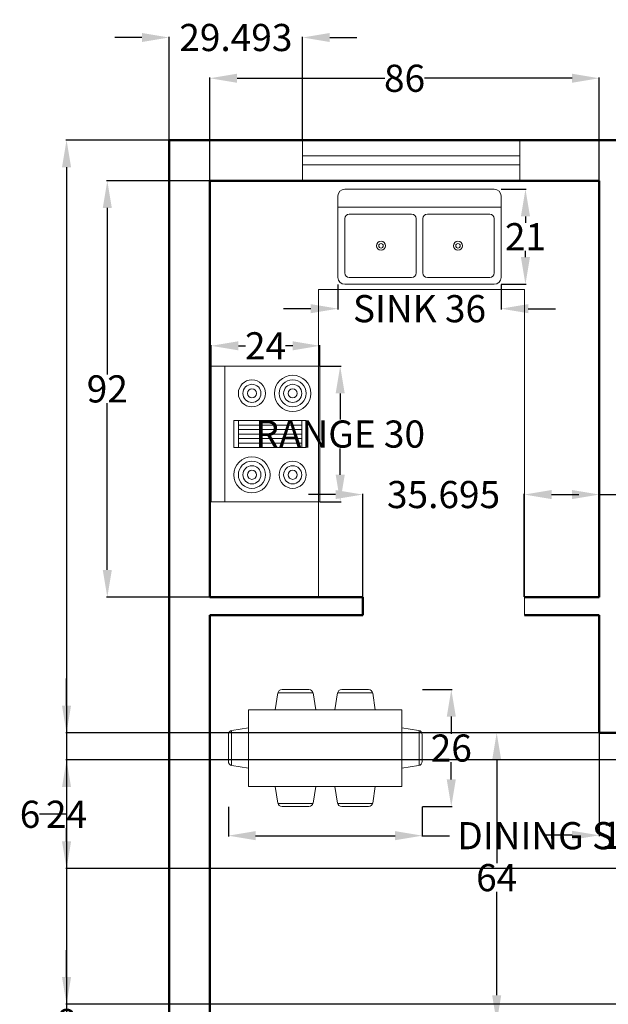
# Model space of a CAD drawing. Units: inches. Extents: x -8 to 300, y -428 to 46.
# Tile 3 of 4: x -8 to 122, y -172 to 46. Entities that reach past the tile are written whole.
import ezdxf

# ---------------------------------------------------------------- set-up
doc = ezdxf.new("R2010")
doc.units = ezdxf.units.IN
doc.header["$MEASUREMENT"] = 0
for name, color, linetype, lineweight in [('A-ANNO-DIMS', 2, 'Continuous', 18), ('A-EQPM', 8, 'Continuous', 18), ('A-FLOR-CASE', 9, 'Continuous', 18), ('A-FLOR-FIXT', 9, 'Continuous', 18), ('A-FURN', 8, 'Continuous', 18), ('A-GLAZ', 4, 'Continuous', 18), ('A-WALL', 7, 'Continuous', 50)]:
    doc.layers.add(name, color=color, linetype=linetype, lineweight=lineweight)
doc.styles.get("Standard").update_dxf_attribs({"font": 'arial.ttf'})
doc.dimstyles.get("Standard").update_dxf_attribs({"dimtxt": 6, "dimasz": 6, "dimexe": 0.18, "dimexo": 0.0625, "dimgap": 0.09, "dimtad": 0, "dimtih": 1, "dimtoh": 1, "dimdec": 0, "dimzin": 0, "dimdsep": 46, "dimlunit": 4, "dimtxsty": 'Standard', "dimcen": 0.09, "dimadec": 0, "dimazin": 0, "dimtfac": 1, "dimtdec": 0, "dimtofl": 0, "dimtmove": 0, "dimatfit": 3, "dimfxl": 1, "dimtolj": 1, "dimtzin": 0, "dimarcsym": 0})

# ---------------------------------------------------------------- blocks, each defined once
blk = doc.blocks.new('Dining Set - 36 x 72 in.')
for p, q in [((-22.23, 26), (-23.48, 18)), ((-22.23, 26), (-5.76, 26)), ((-5.84, 26.5), (-5.84, 26.5)), ((-4.52, 18), (-5.77, 26)), ((5.77, 26), (4.52, 18)), ((5.77, 26), (22.24, 26)), ((22.16, 26.5), (22.16, 26.5)), ((36, 18), (-36, 18)), ((-36, 18), (-36, -18)), ((36, -18), (36, 18)), ((-43.81, 8.26), (-36, 9.48)), ((43.81, 8.26), (36, 9.48)), ((-45.5, 6.29), (-45.5, -6.29)), ((-44, 8.23), (-44, -8.24)), ((44, 8.23), (44, -8.24)), ((45.5, 6.29), (45.5, -6.29)), ((-44.5, -8.16), (-44.5, -8.16)), ((-36, -9.48), (-43.81, -8.26)), ((36, -9.48), (43.81, -8.26)), ((44.5, -8.16), (44.5, -8.16)), ((-36, -18), (36, -18)), ((-22.26, -25.81), (-23.48, -18)), ((-4.52, -18), (-5.74, -25.81)), ((5.74, -25.81), (4.52, -18)), ((23.48, -18), (22.26, -25.81)), ((-22.23, -26), (-5.76, -26)), ((-20.29, -27.5), (-7.71, -27.5)), ((-5.84, -26.5), (-5.84, -26.5)), ((5.77, -26), (22.24, -26)), ((7.71, -27.5), (20.29, -27.5)), ((22.16, -26.5), (22.16, -26.5))]:
    blk.add_line(p, q)
for points in [[(-5.77, 26), (-5.74, 25.81, 0.369509), (-7.71, 27.5), (-20.28, 27.5, 0.370247), (-22.26, 25.8), (-22.23, 26)], [(5.7, 25.61), (5.74, 25.81, -0.369509), (7.71, 27.5), (20.29, 27.5, -0.36951), (22.26, 25.81), (23.48, 18)]]:
    blk.add_lwpolyline(points, format="xyb")
for centre, start, end in [((-43.5, 6.29), 98.8806, 180), ((43.5, 6.29), 0, 81.1194), ((-43.5, -6.29), 180, 261.1194), ((43.5, -6.29), 278.8806, 0), ((-20.29, -25.5), 188.8802, 270), ((-7.71, -25.5), 270, 351.1191), ((7.71, -25.5), 188.8802, 270), ((20.29, -25.5), 270, 351.1191)]:
    blk.add_arc(centre, 2, start, end)
blk = doc.blocks.new('Range-Oven - 30 in top')
for p, q in [((0, -3), (30, -3)), ((12, -6), (18, -6)), ((13, -20), (13, -6)), ((14, -6), (14, -20)), ((15, -20), (15, -6)), ((16, -6), (16, -20)), ((17, -20), (17, -6)), ((18, -20), (12, -20))]:
    blk.add_line(p, q)
for points in [[(0, -24), (0, 0), (30, 0), (30, -24)], [(12, -21), (12, -5), (18, -5), (18, -21)]]:
    blk.add_lwpolyline(points, close=True)
for centre, radius in [((6, -9), 4), ((6, -9), 3), ((24, -9), 3), ((6, -9), 2), ((6, -9), 1), ((24, -9), 2), ((24, -9), 1), ((6, -18), 3), ((24, -18), 4), ((24, -18), 3), ((6, -18), 2), ((6, -18), 1), ((24, -18), 2), ((24, -18), 1)]:
    blk.add_circle(centre, radius)
blk = doc.blocks.new('Sink-double - 36 in top')
for p, q in [((-18, -4), (18, -4)), ((-0.75, -18.5), (-0.75, -6.5)), ((0.75, -6.5), (0.75, -18.5))]:
    blk.add_line(p, q)
for points in [[(-16.5, 0), (16.5, 0)], [(-18, -19.5), (-18, -1.5)], [(18, -1.5), (18, -19.5)], [(-16.5, -18.5), (-16.5, -6.5)], [(-15.5, -5.5), (-1.75, -5.5)], [(1.75, -5.5), (15.5, -5.5)], [(16.5, -6.5), (16.5, -18.5)], [(-1.75, -19.5), (-15.5, -19.5)], [(15.5, -19.5), (1.75, -19.5)], [(16.5, -21), (-16.5, -21)]]:
    blk.add_lwpolyline(points)
for centre, radius in [((-8.5, -12.5), 1), ((-8.5, -12.5), 0.5), ((8.5, -12.5), 1), ((8.5, -12.5), 0.5)]:
    blk.add_circle(centre, radius)
for centre, radius, start, end in [((-16.5, -1.5), 1.5, 90, 180), ((16.5, -1.5), 1.5, 0, 90), ((-15.5, -6.5), 1, 90, 180), ((-1.75, -6.5), 1, 0, 90), ((1.75, -6.5), 1, 90, 180), ((15.5, -6.5), 1, 0, 90), ((-16.5, -19.5), 1.5, 180, 270), ((-15.5, -18.5), 1, 180, 270), ((-1.75, -18.5), 1, 270, 0), ((1.75, -18.5), 1, 180, 270), ((15.5, -18.5), 1, 270, 0), ((16.5, -19.5), 1.5, 270, 0)]:
    blk.add_arc(centre, radius, start, end)
blk = doc.blocks.new('*D23')
at = {"layer": 'A-ANNO-DIMS', "color": 0, "lineweight": -2, "transparency": 16777216}
for p, q in [((37.97, -128.08), (37.97, -134.62)), ((80.78, -128.08), (80.78, -134.62)), ((43.97, -134.44), (74.78, -134.44)), ((80.78, -134.44), (86.78, -134.44))]:
    blk.add_line(p, q, dxfattribs=at)
at = {"layer": 'A-ANNO-DIMS', "color": 0, "transparency": 16777216}
for points in [[(43.97, -133.44), (43.97, -135.44), (37.97, -134.44)], [(74.78, -133.44), (74.78, -135.44), (80.78, -134.44)]]:
    blk.add_solid(points, dxfattribs=at)
at = {"layer": 'Defpoints', "color": 0, "transparency": 16777216}
for p in [(37.97, -128.02), (80.78, -128.02), (80.78, -134.44)]:
    blk.add_point(p, dxfattribs=at)
at = {"layer": 'A-ANNO-DIMS', "color": 0, "transparency": 16777216, "insert": (116.16, -134.44), "char_height": 6, "attachment_point": 5}
blk.add_mtext('\\A1;DINING SET 43', dxfattribs=at)
blk = doc.blocks.new('*D24')
at = {"layer": 'A-ANNO-DIMS', "color": 0, "lineweight": -2, "transparency": 16777216}
for p, q in [((80.84, -102.14), (87.38, -102.14)), ((87.2, -108.14), (87.2, -111.93)), ((87.2, -122.02), (87.2, -118.23)), ((80.84, -128.02), (87.38, -128.02))]:
    blk.add_line(p, q, dxfattribs=at)
at = {"layer": 'A-ANNO-DIMS', "color": 0, "transparency": 16777216}
for points in [[(86.2, -108.14), (88.2, -108.14), (87.2, -102.14)], [(86.2, -122.02), (88.2, -122.02), (87.2, -128.02)]]:
    blk.add_solid(points, dxfattribs=at)
at = {"layer": 'Defpoints', "color": 0, "transparency": 16777216}
for p in [(80.78, -102.14), (87.2, -102.14), (80.78, -128.02)]:
    blk.add_point(p, dxfattribs=at)
at = {"layer": 'A-ANNO-DIMS', "color": 0, "transparency": 16777216, "insert": (87.2, -115.08), "char_height": 6, "attachment_point": 5}
blk.add_mtext('\\A1;26', dxfattribs=at)
blk = doc.blocks.new('*D25')
at = {"layer": 'A-ANNO-DIMS', "color": 0, "lineweight": -2, "transparency": 16777216}
for p, q in [((58.23, -30.69), (62.85, -30.69)), ((62.67, -36.69), (62.67, -42.5)), ((62.67, -54.69), (62.67, -48.89)), ((58.23, -60.69), (62.85, -60.69))]:
    blk.add_line(p, q, dxfattribs=at)
at = {"layer": 'A-ANNO-DIMS', "color": 0, "transparency": 16777216}
for points in [[(61.67, -36.69), (63.67, -36.69), (62.67, -30.69)], [(61.67, -54.69), (63.67, -54.69), (62.67, -60.69)]]:
    blk.add_solid(points, dxfattribs=at)
at = {"layer": 'Defpoints', "color": 0, "transparency": 16777216}
for p in [(58.17, -30.69), (62.67, -30.69), (58.17, -60.69)]:
    blk.add_point(p, dxfattribs=at)
at = {"layer": 'A-ANNO-DIMS', "color": 0, "transparency": 16777216, "insert": (62.67, -45.69), "char_height": 6, "attachment_point": 5}
blk.add_mtext('\\A1;RANGE 30', dxfattribs=at)
blk = doc.blocks.new('*D26')
at = {"layer": 'A-ANNO-DIMS', "color": 0, "lineweight": -2, "transparency": 16777216}
for p, q in [((34.17, -30.63), (34.17, -26.01)), ((58.17, -30.63), (58.17, -26.01)), ((40.17, -26.19), (41.75, -26.19)), ((52.17, -26.19), (50.6, -26.19))]:
    blk.add_line(p, q, dxfattribs=at)
at = {"layer": 'A-ANNO-DIMS', "color": 0, "transparency": 16777216}
for points in [[(40.17, -25.19), (40.17, -27.19), (34.17, -26.19)], [(52.17, -25.19), (52.17, -27.19), (58.17, -26.19)]]:
    blk.add_solid(points, dxfattribs=at)
at = {"layer": 'Defpoints', "color": 0, "transparency": 16777216}
for p in [(34.17, -26.19), (34.17, -30.69), (58.17, -30.69)]:
    blk.add_point(p, dxfattribs=at)
at = {"layer": 'A-ANNO-DIMS', "color": 0, "transparency": 16777216, "insert": (46.17, -26.19), "char_height": 6, "attachment_point": 5}
blk.add_mtext('\\A1;24', dxfattribs=at)
blk = doc.blocks.new('*D27')
at = {"layer": 'A-ANNO-DIMS', "color": 0, "lineweight": -2, "transparency": 16777216}
for p, q in [((62.18, -12.64), (62.18, -18.16)), ((98.18, -12.64), (98.18, -18.16)), ((56.18, -17.98), (50.18, -17.98)), ((104.18, -17.98), (110.18, -17.98))]:
    blk.add_line(p, q, dxfattribs=at)
at = {"layer": 'A-ANNO-DIMS', "color": 0, "transparency": 16777216}
for points in [[(56.18, -16.98), (56.18, -18.98), (62.18, -17.98)], [(104.18, -16.98), (104.18, -18.98), (98.18, -17.98)]]:
    blk.add_solid(points, dxfattribs=at)
at = {"layer": 'Defpoints', "color": 0, "transparency": 16777216}
for p in [(62.18, -12.58), (98.18, -12.58), (98.18, -17.98)]:
    blk.add_point(p, dxfattribs=at)
at = {"layer": 'A-ANNO-DIMS', "color": 0, "transparency": 16777216, "insert": (80.18, -17.98), "char_height": 6, "attachment_point": 5}
blk.add_mtext('\\A1;SINK 36', dxfattribs=at)
blk = doc.blocks.new('*D28')
at = {"layer": 'A-ANNO-DIMS', "color": 0, "lineweight": -2, "transparency": 16777216}
for p, q in [((98.24, 8.42), (103.76, 8.42)), ((103.58, 2.42), (103.58, 1.02)), ((103.58, -6.58), (103.58, -5.18)), ((98.24, -12.58), (103.76, -12.58))]:
    blk.add_line(p, q, dxfattribs=at)
at = {"layer": 'A-ANNO-DIMS', "color": 0, "transparency": 16777216}
for points in [[(102.58, 2.42), (104.58, 2.42), (103.58, 8.42)], [(102.58, -6.58), (104.58, -6.58), (103.58, -12.58)]]:
    blk.add_solid(points, dxfattribs=at)
at = {"layer": 'Defpoints', "color": 0, "transparency": 16777216}
for p in [(98.18, 8.42), (103.58, 8.42), (98.18, -12.58)]:
    blk.add_point(p, dxfattribs=at)
at = {"layer": 'A-ANNO-DIMS', "color": 0, "transparency": 16777216, "insert": (103.58, -2.08), "char_height": 6, "attachment_point": 5}
blk.add_mtext('\\A1;21', dxfattribs=at)
blk = doc.blocks.new('*D32')
at = {"layer": 'A-ANNO-DIMS', "color": 0, "lineweight": -2, "transparency": 16777216}
for p, q in [((24.81, 19.29), (2.05, 19.29)), ((2.23, 13.29), (2.23, -187.98)), ((2.23, -395.57), (2.23, -194.29)), ((81.13, -401.57), (2.05, -401.57))]:
    blk.add_line(p, q, dxfattribs=at)
at = {"layer": 'A-ANNO-DIMS', "color": 0, "transparency": 16777216}
for points in [[(1.23, 13.29), (3.23, 13.29), (2.23, 19.29)], [(1.23, -395.57), (3.23, -395.57), (2.23, -401.57)]]:
    blk.add_solid(points, dxfattribs=at)
at = {"layer": 'Defpoints', "color": 0, "transparency": 16777216}
for p in [(24.88, 19.29), (2.23, -401.57), (81.19, -401.57)]:
    blk.add_point(p, dxfattribs=at)
at = {"layer": 'A-ANNO-DIMS', "color": 0, "transparency": 16777216, "insert": (2.23, -191.14), "char_height": 6, "attachment_point": 5}
blk.add_mtext('\\A1;420.9', dxfattribs=at)
blk = doc.blocks.new('*D36')
at = {"layer": 'A-ANNO-DIMS', "color": 0, "lineweight": -2, "transparency": 16777216}
for p, q in [((33.88, 10.36), (33.88, 33.12)), ((39.88, 32.94), (72.49, 32.94)), ((113.88, 32.94), (81.27, 32.94)), ((119.88, 10.36), (119.88, 33.12))]:
    blk.add_line(p, q, dxfattribs=at)
at = {"layer": 'A-ANNO-DIMS', "color": 0, "transparency": 16777216}
for points in [[(39.88, 33.94), (39.88, 31.94), (33.88, 32.94)], [(113.88, 33.94), (113.88, 31.94), (119.88, 32.94)]]:
    blk.add_solid(points, dxfattribs=at)
at = {"layer": 'Defpoints', "color": 0, "transparency": 16777216}
for p in [(119.88, 32.94), (33.88, 10.29), (119.88, 10.29)]:
    blk.add_point(p, dxfattribs=at)
at = {"layer": 'A-ANNO-DIMS', "color": 0, "transparency": 16777216, "insert": (76.88, 32.94), "char_height": 6, "attachment_point": 5}
blk.add_mtext('\\A1;86', dxfattribs=at)
blk = doc.blocks.new('*D38')
at = {"layer": 'A-ANNO-DIMS', "color": 0, "lineweight": -2, "transparency": 16777216}
for p, q in [((33.81, 10.29), (11.05, 10.29)), ((11.23, 4.29), (11.23, -32.55)), ((11.23, -75.71), (11.23, -38.86)), ((33.81, -81.71), (11.05, -81.71))]:
    blk.add_line(p, q, dxfattribs=at)
at = {"layer": 'A-ANNO-DIMS', "color": 0, "transparency": 16777216}
for points in [[(10.23, 4.29), (12.23, 4.29), (11.23, 10.29)], [(10.23, -75.71), (12.23, -75.71), (11.23, -81.71)]]:
    blk.add_solid(points, dxfattribs=at)
at = {"layer": 'Defpoints', "color": 0, "transparency": 16777216}
for p in [(11.23, 10.29), (33.88, 10.29), (33.88, -81.71)]:
    blk.add_point(p, dxfattribs=at)
at = {"layer": 'A-ANNO-DIMS', "color": 0, "transparency": 16777216, "insert": (11.23, -35.71), "char_height": 6, "attachment_point": 5}
blk.add_mtext('\\A1;92', dxfattribs=at)
blk = doc.blocks.new('*D41')
at = {"layer": 'A-ANNO-DIMS', "color": 0, "lineweight": -2, "transparency": 16777216}
for p, q in [((119.81, -111.71), (97.05, -111.71)), ((97.23, -117.71), (97.23, -140.55)), ((97.23, -169.71), (97.23, -146.86)), ((119.81, -175.71), (97.05, -175.71))]:
    blk.add_line(p, q, dxfattribs=at)
at = {"layer": 'A-ANNO-DIMS', "color": 0, "transparency": 16777216}
for points in [[(96.23, -117.71), (98.23, -117.71), (97.23, -111.71)], [(96.23, -169.71), (98.23, -169.71), (97.23, -175.71)]]:
    blk.add_solid(points, dxfattribs=at)
at = {"layer": 'Defpoints', "color": 0, "transparency": 16777216}
for p in [(97.23, -111.71), (119.88, -111.71), (119.88, -175.71)]:
    blk.add_point(p, dxfattribs=at)
at = {"layer": 'A-ANNO-DIMS', "color": 0, "transparency": 16777216, "insert": (97.23, -143.71), "char_height": 6, "attachment_point": 5}
blk.add_mtext('\\A1;64', dxfattribs=at)
blk = doc.blocks.new('*D45')
at = {"layer": 'A-ANNO-DIMS', "color": 0, "lineweight": -2, "transparency": 16777216}
for p, q in [((119.875934, -111.769234), (119.875934, -134.536734)), ((129.875934, -111.769234), (129.875934, -134.536734)), ((113.875934, -134.356734), (107.875934, -134.356734)), ((135.875934, -134.356734), (141.875934, -134.356734))]:
    blk.add_line(p, q, dxfattribs=at)
at = {"layer": 'A-ANNO-DIMS', "color": 0, "transparency": 16777216}
for points in [[(113.875934, -133.356734), (113.875934, -135.356734), (119.875934, -134.356734)], [(135.875934, -133.356734), (135.875934, -135.356734), (129.875934, -134.356734)]]:
    blk.add_solid(points, dxfattribs=at)
at = {"layer": 'Defpoints', "color": 0, "transparency": 16777216}
for p in [(119.875934, -111.706734), (129.875934, -111.706734), (119.875934, -134.356734)]:
    blk.add_point(p, dxfattribs=at)
at = {"layer": 'A-ANNO-DIMS', "color": 0, "transparency": 16777216, "insert": (124.875934, -134.356734), "char_height": 6, "attachment_point": 5}
blk.add_mtext('\\A1;10', dxfattribs=at)
blk = doc.blocks.new('*D46')
at = {"layer": 'A-ANNO-DIMS', "color": 0, "lineweight": -2, "transparency": 16777216}
for p, q in [((61.64046, -59.056734), (55.64046, -59.056734)), ((67.64046, -81.644234), (67.64046, -58.876734)), ((103.334962, -81.644234), (103.334962, -58.876734)), ((109.334962, -59.056734), (115.334962, -59.056734))]:
    blk.add_line(p, q, dxfattribs=at)
at = {"layer": 'A-ANNO-DIMS', "color": 0, "transparency": 16777216}
for points in [[(61.64046, -58.056734), (61.64046, -60.056734), (67.64046, -59.056734)], [(109.334962, -58.056734), (109.334962, -60.056734), (103.334962, -59.056734)]]:
    blk.add_solid(points, dxfattribs=at)
at = {"layer": 'Defpoints', "color": 0, "transparency": 16777216}
for p in [(103.334962, -59.056734), (67.64046, -81.706734), (103.334962, -81.706734)]:
    blk.add_point(p, dxfattribs=at)
at = {"layer": 'A-ANNO-DIMS', "color": 0, "transparency": 16777216, "insert": (85.487711, -59.056734), "char_height": 6, "attachment_point": 5}
blk.add_mtext('\\A1;35.695', dxfattribs=at)
blk = doc.blocks.new('*D47')
at = {"layer": 'A-ANNO-DIMS', "color": 0, "lineweight": -2, "transparency": 16777216}
for p, q in [((103.33, -81.64), (103.33, -58.88)), ((109.33, -59.06), (113.88, -59.06)), ((119.88, -81.64), (119.88, -58.88)), ((119.88, -59.06), (125.88, -59.06))]:
    blk.add_line(p, q, dxfattribs=at)
at = {"layer": 'A-ANNO-DIMS', "color": 0, "transparency": 16777216}
for points in [[(109.33, -58.06), (109.33, -60.06), (103.33, -59.06)], [(113.88, -58.06), (113.88, -60.06), (119.88, -59.06)]]:
    blk.add_solid(points, dxfattribs=at)
at = {"layer": 'Defpoints', "color": 0, "transparency": 16777216}
for p in [(119.88, -59.06), (103.33, -81.71), (119.88, -81.71)]:
    blk.add_point(p, dxfattribs=at)
at = {"layer": 'A-ANNO-DIMS', "color": 0, "transparency": 16777216, "insert": (135.79, -59.06), "char_height": 6, "attachment_point": 5}
blk.add_mtext('\\A1;16.54', dxfattribs=at)
blk = doc.blocks.new('*D48')
at = {"layer": 'A-ANNO-DIMS', "color": 0, "lineweight": -2, "transparency": 16777216}
for p, q in [((18.875934, 41.943266), (12.875934, 41.943266)), ((24.875934, 19.355766), (24.875934, 42.123266)), ((54.36899, 19.355766), (54.36899, 42.123266)), ((60.36899, 41.943266), (66.36899, 41.943266))]:
    blk.add_line(p, q, dxfattribs=at)
at = {"layer": 'A-ANNO-DIMS', "color": 0, "transparency": 16777216}
for points in [[(18.875934, 42.943266), (18.875934, 40.943266), (24.875934, 41.943266)], [(60.36899, 42.943266), (60.36899, 40.943266), (54.36899, 41.943266)]]:
    blk.add_solid(points, dxfattribs=at)
at = {"layer": 'Defpoints', "color": 0, "transparency": 16777216}
for p in [(54.36899, 41.943266), (24.875934, 19.293266), (54.36899, 19.293266)]:
    blk.add_point(p, dxfattribs=at)
at = {"layer": 'A-ANNO-DIMS', "color": 0, "transparency": 16777216, "insert": (39.622462, 41.943266), "char_height": 6, "attachment_point": 5}
blk.add_mtext('\\A1;29.493', dxfattribs=at)
blk = doc.blocks.new('*D56')
at = {"layer": 'A-ANNO-DIMS', "color": 0, "lineweight": -2, "transparency": 16777216}
for p, q in [((177.81, -117.71), (2.05, -117.71)), ((2.23, -123.71), (2.23, -126.6)), ((2.23, -135.71), (2.23, -132.81)), ((177.81, -141.71), (2.05, -141.71))]:
    blk.add_line(p, q, dxfattribs=at)
at = {"layer": 'A-ANNO-DIMS', "color": 0, "transparency": 16777216}
for points in [[(1.23, -123.71), (3.23, -123.71), (2.23, -117.71)], [(1.23, -135.71), (3.23, -135.71), (2.23, -141.71)]]:
    blk.add_solid(points, dxfattribs=at)
at = {"layer": 'Defpoints', "color": 0, "transparency": 16777216}
for p in [(177.88, -117.71), (2.23, -141.71), (177.88, -141.71)]:
    blk.add_point(p, dxfattribs=at)
at = {"layer": 'A-ANNO-DIMS', "color": 0, "transparency": 16777216, "insert": (2.23, -129.71), "char_height": 6, "attachment_point": 5}
blk.add_mtext('\\A1;24', dxfattribs=at)
blk = doc.blocks.new('*D57')
at = {"layer": 'A-ANNO-DIMS', "color": 0, "lineweight": -2, "transparency": 16777216}
for p, q in [((2.23, -105.71), (2.23, -99.71)), ((177.81, -111.71), (2.05, -111.71)), ((177.81, -117.71), (2.05, -117.71)), ((2.23, -123.71), (2.23, -129.71)), ((2.23, -129.71), (-3.77, -129.71))]:
    blk.add_line(p, q, dxfattribs=at)
at = {"layer": 'A-ANNO-DIMS', "color": 0, "transparency": 16777216}
for points in [[(1.23, -105.71), (3.23, -105.71), (2.23, -111.71)], [(1.23, -123.71), (3.23, -123.71), (2.23, -117.71)]]:
    blk.add_solid(points, dxfattribs=at)
at = {"layer": 'Defpoints', "color": 0, "transparency": 16777216}
for p in [(177.88, -111.71), (2.23, -117.71), (177.88, -117.71)]:
    blk.add_point(p, dxfattribs=at)
at = {"layer": 'A-ANNO-DIMS', "color": 0, "transparency": 16777216, "insert": (-5.84, -129.71), "char_height": 6, "attachment_point": 5}
blk.add_mtext('\\A1;6', dxfattribs=at)
blk = doc.blocks.new('*D58')
at = {"layer": 'A-ANNO-DIMS', "color": 0, "lineweight": -2, "transparency": 16777216}
for p, q in [((2.225934, -165.706734), (2.225934, -159.706734)), ((181.813434, -171.706734), (2.045934, -171.706734)), ((177.813434, -179.706734), (2.045934, -179.706734)), ((2.225934, -185.706734), (2.225934, -191.706734))]:
    blk.add_line(p, q, dxfattribs=at)
at = {"layer": 'A-ANNO-DIMS', "color": 0, "transparency": 16777216}
for points in [[(1.225934, -165.706734), (3.225934, -165.706734), (2.225934, -171.706734)], [(1.225934, -185.706734), (3.225934, -185.706734), (2.225934, -179.706734)]]:
    blk.add_solid(points, dxfattribs=at)
at = {"layer": 'Defpoints', "color": 0, "transparency": 16777216}
for p in [(2.225934, -171.706734), (181.875934, -171.706734), (177.875934, -179.706734)]:
    blk.add_point(p, dxfattribs=at)
at = {"layer": 'A-ANNO-DIMS', "color": 0, "transparency": 16777216, "insert": (2.225934, -175.706734), "char_height": 6, "attachment_point": 5}
blk.add_mtext('\\A1;8', dxfattribs=at)

msp = doc.modelspace()

# ---------------------------------------------------------------- linework, layer by layer
at = {"layer": 'A-FLOR-CASE'}
for p, q in [((57.8759, -81.7067), (57.8759, -13.7067)), ((57.8759, -13.7067), (103.335, -13.7067)), ((103.335, -13.7067), (103.335, -85.7067))]:
    msp.add_line(p, q, dxfattribs=at)
at = {"layer": 'A-GLAZ'}
for p, q in [((54.369, 10.2933), (54.369, 19.2933)), ((102.369, 19.2996), (102.369, 10.2933)), ((54.369, 15.7933), (102.369, 15.7933)), ((54.369, 13.7933), (102.369, 13.7933))]:
    msp.add_line(p, q, dxfattribs=at)
at = {"layer": 'A-WALL'}
for p, q in [((33.8759, 10.2933), (119.8759, 10.2933)), ((33.8759, -81.7067), (33.8759, 10.2933)), ((119.8759, 10.2933), (119.8759, -81.7067)), ((33.8759, -81.7067), (67.6405, -81.7067)), ((67.6405, -81.7067), (67.6405, -85.7067)), ((103.335, -81.7067), (119.8759, -81.7067)), ((33.8759, -331.7067), (33.8759, -85.7067)), ((33.8759, -85.7067), (67.6405, -85.7067)), ((103.335, -85.7067), (119.8759, -85.7067)), ((119.8759, -85.7067), (119.8759, -111.7067)), ((119.8759, -111.7067), (129.8759, -111.7067))]:
    msp.add_line(p, q, dxfattribs=at)
msp.add_lwpolyline([(39.8759, -340.7067), (24.8759, -340.7067), (24.8759, 19.2933), (264.8759, 19.2933), (264.8759, -340.7067), (197.0947, -340.7067)], dxfattribs=at)

# ---------------------------------------------------------------- block references
at = {"layer": 'A-EQPM', "rotation": 90}
msp.add_blockref('Range-Oven - 30 in top', (34.1716, -60.6947), dxfattribs=at)
at = {"layer": 'A-FLOR-FIXT'}
msp.add_blockref('Sink-double - 36 in top', (80.1795, 8.4213), dxfattribs=at)
at = {"layer": 'A-FURN', "xscale": 0.4704014302030969, "yscale": 0.4704014302030969, "zscale": 0.4704014302030969}
msp.add_blockref('Dining Set - 36 x 72 in.', (59.3744, -115.0796), dxfattribs=at)

# ---------------------------------------------------------------- dimensions: what is measured, and where the dimension line sits
at = {"layer": 'A-ANNO-DIMS'}
for base, p1, p2, angle, override, picture, middle in [((54.369, 41.9433), (24.8759, 19.2933), (54.369, 19.2933), 0, {"dimdec": 3, "dimlfac": 1, "dimrnd": 0, "dimzin": 0, "dimdsep": 46, "dimlunit": 2}, '*D48', (39.6225, 41.9433)), ((119.8759, 32.9433), (33.8759, 10.2933), (119.8759, 10.2933), 0, {"dimdec": 0, "dimlfac": 1, "dimrnd": 0, "dimzin": 0, "dimdsep": 46, "dimlunit": 2}, '*D36', (76.8759, 32.9433)), ((2.2259, -401.5677), (24.8759, 19.2933), (81.1915, -401.5677), 90, {"dimdec": 1, "dimlfac": 1, "dimrnd": 0, "dimzin": 0, "dimdsep": 46, "dimlunit": 2}, '*D32', (2.2259, -191.1372)), ((11.2259, 10.2933), (33.8759, -81.7067), (33.8759, 10.2933), 90, {"dimdec": 0, "dimlfac": 1, "dimrnd": 0, "dimzin": 0, "dimdsep": 46, "dimlunit": 2}, '*D38', (11.2259, -35.7067)), ((103.5795, 8.4213), (98.1795, -12.5787), (98.1795, 8.4213), 90, {"dimdec": 0, "dimlfac": 1, "dimrnd": 0, "dimzin": 0, "dimdsep": 46, "dimlunit": 2}, '*D28', (103.5795, -2.0787)), ((34.1716, -26.1947), (58.1716, -30.6947), (34.1716, -30.6947), 180, {"dimdec": 0, "dimlfac": 1, "dimrnd": 0, "dimzin": 0, "dimdsep": 46, "dimlunit": 2}, '*D26', (46.1716, -26.1947)), ((2.2259, -117.7067), (177.8759, -111.7067), (177.8759, -117.7067), 90, {"dimdec": 0, "dimlfac": 1, "dimrnd": 0, "dimzin": 0, "dimdsep": 46, "dimlunit": 2}, '*D57', (-5.845, -129.7067)), ((87.1986, -102.1435), (80.7776, -128.0156), (80.7776, -102.1435), 90, {"dimdec": 0, "dimlfac": 1, "dimrnd": 0, "dimzin": 0, "dimdsep": 46, "dimlunit": 2}, '*D24', (87.1986, -115.0796)), ((97.2259, -111.7067), (119.8759, -175.7067), (119.8759, -111.7067), 90, {"dimdec": 0, "dimlfac": 1, "dimrnd": 0, "dimzin": 0, "dimdsep": 46, "dimlunit": 2}, '*D41', (97.2259, -143.7067)), ((119.8759, -134.3567), (129.8759, -111.7067), (119.8759, -111.7067), 180, {"dimdec": 0, "dimlfac": 1, "dimrnd": 0, "dimzin": 0, "dimdsep": 46, "dimlunit": 2}, '*D45', (124.8759, -134.3567)), ((2.2259, -141.7067), (177.8759, -117.7067), (177.8759, -141.7067), 90, {"dimdec": 0, "dimlfac": 1, "dimrnd": 0, "dimzin": 0, "dimdsep": 46, "dimlunit": 2}, '*D56', (2.2259, -129.7067)), ((2.2259, -171.7067), (177.8759, -179.7067), (181.8759, -171.7067), 90, {"dimdec": 0, "dimlfac": 1, "dimrnd": 0, "dimzin": 0, "dimdsep": 46, "dimlunit": 2}, '*D58', (2.2259, -175.7067))]:
    dim = msp.add_linear_dim(base=base, p1=p1, p2=p2, angle=angle, dimstyle='Standard', override=override, dxfattribs=at)
    dim.commit()
    dim.dimension.update_dxf_attribs({"geometry": picture, "text_midpoint": middle})
for base, p1, p2, text, picture, middle in [((98.1795, -17.9787), (62.1795, -12.5787), (98.1795, -12.5787), 'SINK <>', '*D27', (80.1795, -17.9787)), ((80.7776, -134.4366), (37.9711, -128.0156), (80.7776, -128.0156), 'DINING SET <>', '*D23', (116.1637, -134.4366))]:
    dim = msp.add_linear_dim(base=base, p1=p1, p2=p2, text=text, dimstyle='Standard', override={"dimdec": 0, "dimlfac": 1, "dimrnd": 0, "dimzin": 0, "dimdsep": 46, "dimlunit": 2}, dxfattribs=at)
    dim.commit()
    dim.dimension.update_dxf_attribs({"geometry": picture, "text_midpoint": middle})
dim = msp.add_linear_dim(base=(62.6716, -30.6947), p1=(58.1716, -60.6947), p2=(58.1716, -30.6947), angle=90, text='RANGE <>', dimstyle='Standard', override={"dimdec": 0, "dimlfac": 1, "dimrnd": 0, "dimzin": 0, "dimdsep": 46, "dimlunit": 2}, dxfattribs=at)
dim.commit()
dim.dimension.update_dxf_attribs({"geometry": '*D25', "text_midpoint": (62.6716, -45.6947)})
for base, p1, p2, override, picture, middle in [((103.334962, -59.056734), (67.64046, -81.706734), (103.334962, -81.706734), {"dimdec": 3, "dimlfac": 1, "dimrnd": 0, "dimzin": 0, "dimdsep": 46, "dimlunit": 2}, '*D46', (85.487711, -59.056734)), ((119.8759, -59.0567), (103.335, -81.7067), (119.8759, -81.7067), {"dimdec": 2, "dimlfac": 1, "dimrnd": 0, "dimzin": 0, "dimdsep": 46, "dimlunit": 2}, '*D47', (135.7947, -59.0567))]:
    dim = msp.add_linear_dim(base=base, p1=p1, p2=p2, dimstyle='Standard', override=override, dxfattribs=at)
    dim.commit()
    dim.dimension.update_dxf_attribs({"geometry": picture, "text_midpoint": middle})

doc.saveas('drawing.dxf')
